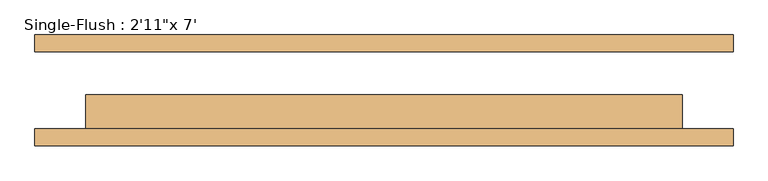
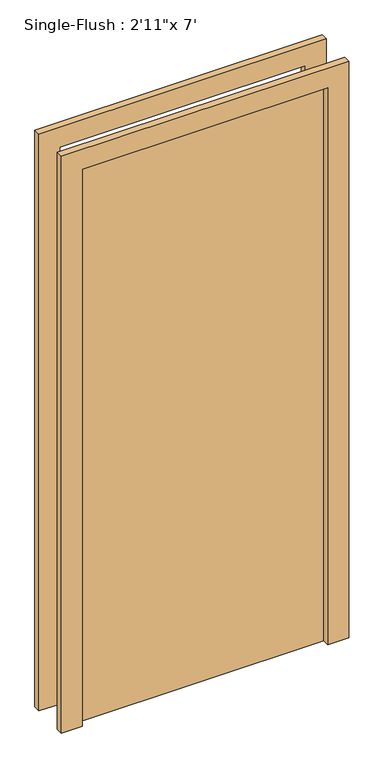
"""IFC4 building model written with IfcOpenShell, lengths in millimetres: door geometry."""

from ifc_helpers import new_model, si_unit, frame, origin, origin_with_axes, place, context, project, spatial, polyline, outline, extrude, source, transform, mapped, element, save


def door_8cb1b8a7(model_context):
    return source(origin(), model_context, "Body", "SweptSolid", [
        extrude(outline(polyline([(2209.8, -520.7), (0.0, -520.7), (0.0, -444.5), (2133.6, -444.5), (2133.6, 444.5), (0.0, 444.5), (0.0, 520.7), (2209.8, 520.7), (2209.8, -520.7)])), frame((0.0, -82.55, 0.0), z_axis=(0.0, 1.0, 0.0), x_axis=(0.0, 0.0, 1.0)), (0.0, 0.0, 1.0), 25.4),
        extrude(outline(polyline([(2209.8, 520.7), (2209.8, -520.7), (0.0, -520.7), (0.0, -444.5), (2133.6, -444.5), (2133.6, 444.5), (0.0, 444.5), (0.0, 520.7), (2209.8, 520.7)])), frame((0.0, 57.15, 0.0), z_axis=(0.0, 1.0, 0.0), x_axis=(0.0, 0.0, 1.0)), (0.0, 0.0, 1.0), 25.4),
        extrude(outline(polyline([(444.5, -6.35), (444.5, -57.15), (-444.5, -57.15), (-444.5, -6.35), (444.5, -6.35)])), origin_with_axes(), (0.0, 0.0, 1.0), 2133.6),
    ])


if __name__ == "__main__":
    model = new_model("IFC4")
    model_context = context("Model", 3, world=origin())
    ifc_project = project(units=[si_unit("LENGTHUNIT", "METRE", prefix="MILLI")], contexts=[model_context])
    site = spatial("IfcSite", under=ifc_project)
    building = spatial("IfcBuilding", under=site)
    placement = place(None, origin())
    door_shape = door_8cb1b8a7(model_context)
    element("IfcDoor", 1, ObjectType="Single-Flush : 2'11\"x 7'", at=placement, inside=building, context=model_context, shape_type="MappedRepresentation", body=[
        mapped(door_shape, transform((0.0, 0.0, 0.0), x_axis=(1.0, 0.0, 0.0), y_axis=(0.0, 1.0, 0.0), z_axis=(0.0, 0.0, 1.0))),
    ])
    save(model, "model.ifc")

# Revit data of these elements
# Type "Single-Flush : 2'11\"x 7'"
#   Type Mark = "12"
#   Construction Type Id = "MDOOR"
#   Assembly Code = "C1020"
#   Analytic Construction = "Metal"
#   Thickness = 0' - 2"
#   Heat Transfer Coefficient (U) = 0.651978 BTU/(h·ft²·°F)
#   Height = 7' - 0"
#   Trim Projection Ext = 0' - 1"
#   Trim Projection Int = 0' - 1"
#   Trim Width = 0' - 3"
#   Width = 2' - 11"
#   Define Thermal Properties by = 1
#   Door Material = Door - Panel
#   Frame Material = Door - Frame
#   Visual Light Transmittance = 0
#   Solar Heat Gain Coefficient = 0
#   Function = (empty or 0)
#   Wall Closure = (empty or 0)
# Element 1 (IfcDoor, "Single-Flush : 2'11\"x 7'")
#   Materials on its faces: "Door - Frame", "Door - Panel"
# Materials
#   "Door - Panel": class "Wood", colour RGB 210 159 95, transparency 0, Cost = 0
#   "Door - Frame": colour RGB 118 70 51, transparency 0, Cost = 0
